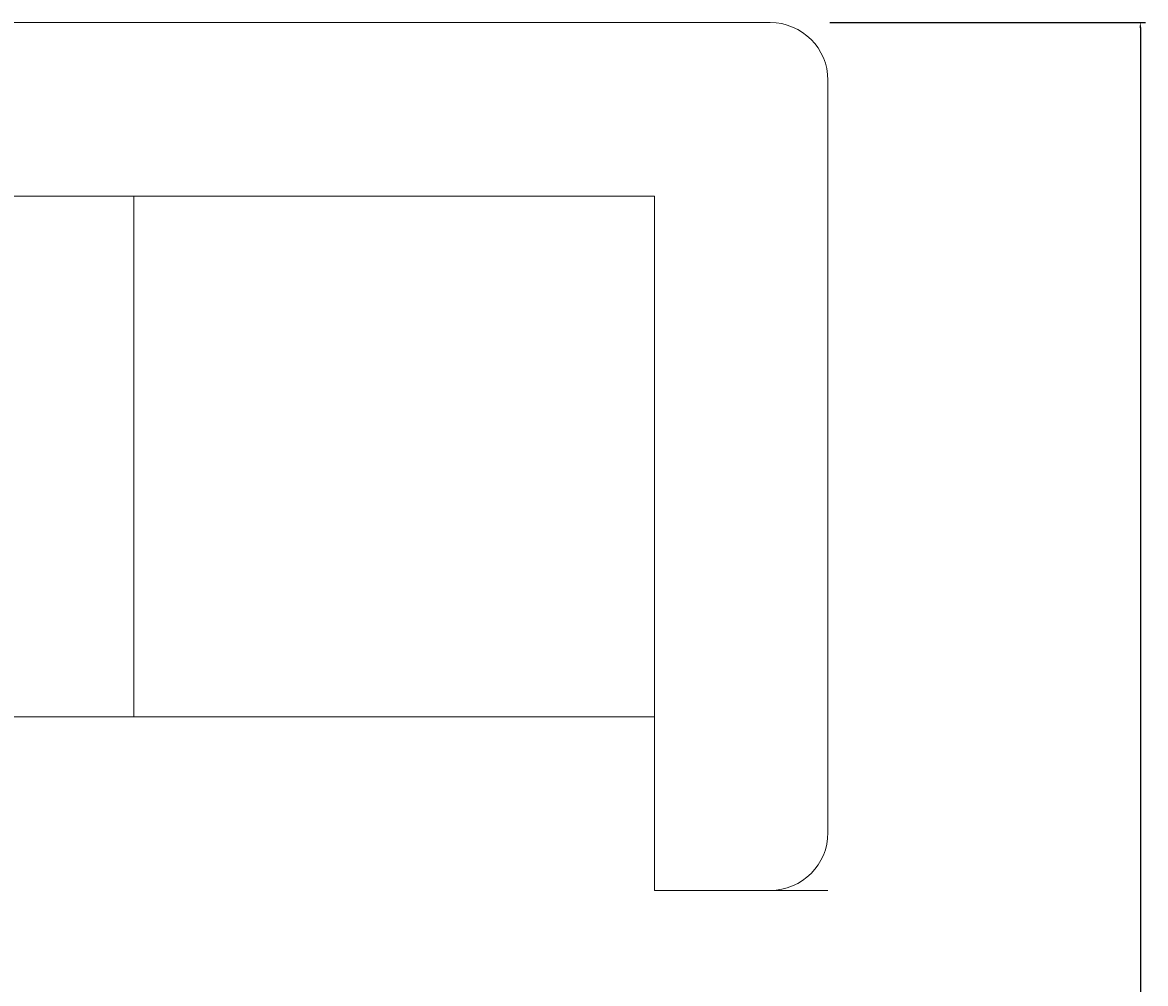
# Model space of a CAD drawing. Units: inches. Extents: x 2307 to 2544, y 2171 to 2540.
# Tile 6 of 52: x 2384 to 2422, y 2247 to 2280. Entities that reach past the tile are written whole.
import ezdxf

# ---------------------------------------------------------------- set-up
doc = ezdxf.new("R2010")
doc.units = ezdxf.units.IN
doc.layers.add('A-ANNO-DIMS', color=2, linetype='Continuous', lineweight=18)
doc.layers.add('A-FURN', color=8, linetype='Continuous', lineweight=18)
doc.styles.get("Standard").update_dxf_attribs({"font": 'arial.ttf'})
doc.dimstyles.get("Standard").update_dxf_attribs({"dimtxt": 0.18, "dimasz": 0.18, "dimexe": 0.18, "dimexo": 0.0625, "dimgap": 0.09, "dimtad": 0, "dimtih": 1, "dimtoh": 1, "dimdec": 4, "dimzin": 0, "dimdsep": 46, "dimtxsty": 'Standard', "dimcen": 0.09, "dimadec": 0, "dimazin": 0, "dimtfac": 1, "dimtdec": 4, "dimtofl": 0, "dimtmove": 0, "dimatfit": 3, "dimfxl": 1, "dimtolj": 1, "dimtzin": 0, "dimarcsym": 0})

# ---------------------------------------------------------------- blocks, each defined once
blk = doc.blocks.new('sofa')
for p, q in [((49, 6), (-19, 6)), ((51, -22), (51, 4)), ((45, -24), (45, 0)), ((45, -24), (49, -24))]:
    blk.add_line(p, q)
blk.add_lwpolyline([(45, 0), (-13, 0, 0.414214), (-15, -2), (-15, -24), (3, -24), (3, -18)], format="xyb")
for points in [[(27, 0), (9, 0), (9, -18), (27, -18)], [(45, 0), (27, 0), (27, -18), (45, -18)]]:
    blk.add_lwpolyline(points, close=True)
for centre, start, end in [((49, 4), 0, 90), ((49, -22), 270, 0)]:
    blk.add_arc(centre, 2, start, end)
blk = doc.blocks.new('*D35')
at = {"layer": 'A-ANNO-DIMS', "color": 0, "lineweight": -2, "transparency": 16777216}
for p, q in [((2411.518, 2280.186), (2422.436, 2280.186)), ((2422.256, 2280.006), (2422.256, 2244.366)), ((2422.256, 2208.366), (2422.256, 2244.005)), ((2411.518, 2208.186), (2422.436, 2208.186))]:
    blk.add_line(p, q, dxfattribs=at)
at = {"layer": 'A-ANNO-DIMS', "color": 0, "transparency": 16777216}
for points in [[(2422.226, 2280.006), (2422.286, 2280.006), (2422.256, 2280.186)], [(2422.226, 2208.366), (2422.286, 2208.366), (2422.256, 2208.186)]]:
    blk.add_solid(points, dxfattribs=at)
at = {"layer": 'Defpoints', "color": 0, "transparency": 16777216}
for p in [(2411.456, 2280.186), (2422.256, 2280.186), (2411.456, 2208.186)]:
    blk.add_point(p, dxfattribs=at)
at = {"layer": 'A-ANNO-DIMS', "color": 0, "transparency": 16777216, "insert": (2422.256, 2244.186), "char_height": 0.18, "attachment_point": 5}
blk.add_mtext('\\A1;72', dxfattribs=at)

msp = doc.modelspace()

# ---------------------------------------------------------------- linework, layer by layer
at = {"layer": 'A-FURN'}
msp.add_line((2405.4557, 2250.1858), (2411.4557, 2250.1858), dxfattribs=at)

# ---------------------------------------------------------------- block references
msp.add_blockref('sofa', (2360.4557, 2274.1858), dxfattribs=at)

# ---------------------------------------------------------------- dimensions: what is measured, and where the dimension line sits
at = {"layer": 'A-ANNO-DIMS'}
dim = msp.add_linear_dim(base=(2422.2557, 2280.1858), p1=(2411.4557, 2208.1858), p2=(2411.4557, 2280.1858), angle=90, dimstyle='Standard', override={"dimdec": 0, "dimlfac": 1, "dimrnd": 0, "dimzin": 0, "dimdsep": 46, "dimlunit": 2}, dxfattribs=at)
dim.commit()
dim.dimension.update_dxf_attribs({"geometry": '*D35', "text_midpoint": (2422.2557, 2244.1858)})

doc.saveas('drawing.dxf')
